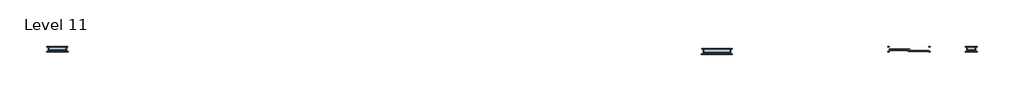
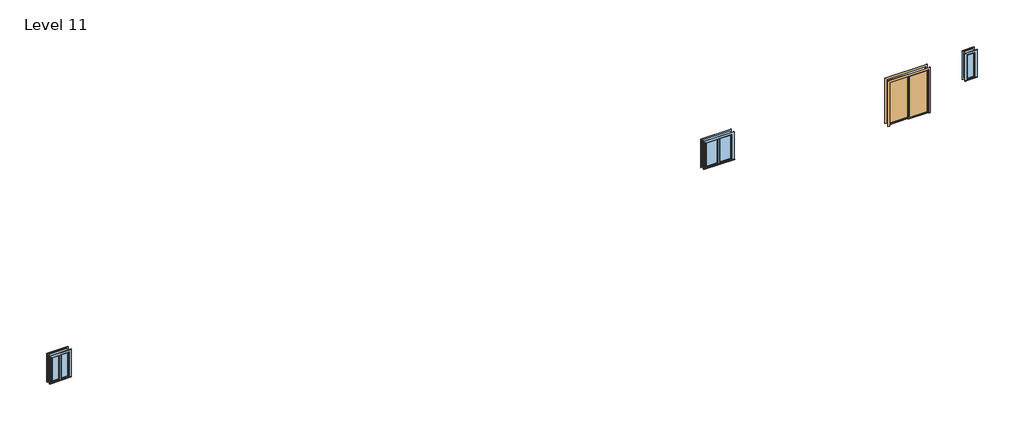
# One storey: 3 windows, 1 door.
"""IFC4 building model written with IfcOpenShell, lengths in millimetres."""

from ifc_helpers import new_model, si_unit, origin, place, context, project, spatial, transform, mapped, element, save
from components import door_076b30e0, window_a765b88f, window_bb17773d, window_0862ab64

model = new_model("IFC4")

# Units and contexts
model_context = context("Model", 3, world=origin())
ifc_project = project(units=[si_unit("LENGTHUNIT", "METRE", prefix="MILLI")], contexts=[model_context])

# Site, building, storey
site = spatial("IfcSite", under=ifc_project)
building = spatial("IfcBuilding", under=site)
storey = spatial("IfcBuildingStorey", under=building, Name="Level 11", Elevation=19507.2)

# Door
placement = place(None, origin())
door_shape = door_076b30e0(model_context)
element("IfcDoor", 1, ObjectType="Door-Double-Sliding : 68\" x 80\"", at=placement, inside=storey, context=model_context, shape_type="MappedRepresentation", body=[
    mapped(door_shape, transform((18530.214721, -12227.7237084, 19507.2), x_axis=(-1.0, 0.0, 0.0), y_axis=(0.0, -1.0, 0.0), z_axis=(0.0, 0.0, 1.0))),
])

# Windows
window_shape = window_a765b88f(model_context)
element("IfcWindow", 2, ObjectType="Awning with Trim : 16\" x 48\"", at=placement, inside=storey, context=model_context, shape_type="MappedRepresentation", body=[
    mapped(window_shape, transform((21273.414721, -12354.7237084, 19507.2), x_axis=(-1.0, 0.0, 0.0), y_axis=(0.0, -1.0, 0.0), z_axis=(0.0, 0.0, 1.0))),
])
window_2_shape = window_bb17773d(model_context)
element("IfcWindow", 3, ObjectType="Casement Dbl with Trim : 32\" x 48\"", at=placement, inside=storey, context=model_context, shape_type="MappedRepresentation", body=[
    mapped(window_2_shape, transform((-18960.185279, -12335.6737084, 19507.2), x_axis=(-1.0, 0.0, 0.0), y_axis=(0.0, -1.0, 0.0), z_axis=(0.0, 0.0, 1.0))),
])
window_3_shape = window_0862ab64(model_context)
element("IfcWindow", 4, ObjectType="Casement Dbl with Trim : 48\" x 48\"", at=placement, inside=storey, context=model_context, shape_type="MappedRepresentation", body=[
    mapped(window_3_shape, transform((10076.7594464, -12437.2737084, 19507.2), x_axis=(-1.0, 0.0, 0.0), y_axis=(0.0, -1.0, 0.0), z_axis=(0.0, 0.0, 1.0))),
])

save(model, "model.ifc")

# Revit data of these elements
# Type "Door-Double-Sliding : 68\" x 80\""
#   Type Mark = "10"
#   Construction Type Id = "opn-d45"
#   Assembly Code = "C1020"
#   Analytic Construction = "Wood frame, double glass door "
#   Thickness = 0' - 2"
#   Thermal Resistance (R) = 1.8150 (h·ft²·°F)/BTU
#   Heat Transfer Coefficient (U) = 0.5510 BTU/(h·ft²·°F)
#   Height = 6' - 8"
#   Rail Width = 0' - 2"
#   Stiles = 0' - 2"
#   Trim Projection Ext = 0' - 1"
#   Trim Projection Int = 0' - 1"
#   Trim Width = 0' - 3"
#   Width = 5' - 8"
#   Define Thermal Properties by = 1
#   Glazing = Glass
#   Panel Material = Wood - Birch - Solid Stained Light Low Gloss
#   Trim Material = Paint - Sienna
#   Visual Light Transmittance = 0
#   Solar Heat Gain Coefficient = 0
#   Function = (empty or 0)
#   Wall Closure = (empty or 0)
# Type "Awning with Trim : 16\" x 48\""
#   Type Mark = "14"
#   Construction Type Id = "GSP4R"
#   Assembly Code = "B2020100"
#   Analytic Construction = "1/8 in Pilkington single glazing"
#   Visual Light Transmittance = 0.9
#   Solar Heat Gain Coefficient = 0.78
#   Heat Transfer Coefficient (U) = 0.6496 BTU/(h·ft²·°F)
#   Height = 4' - 0"
#   Default Sill Height = 3' - 0"
#   Trim Projection - Ext. = 0' - 0 1/2"
#   Trim Projection - Int. = 0' - 0 3/4"
#   Trim Width - Exterior = 0' - 3 1/2"
#   Trim Width - Interior = 0' - 3 1/2"
#   Width = 1' - 4"
#   Window Inset = 0' - 0 3/4"
#   Define Thermal Properties by = 1
#   Glass Pane Material = Glass
#   Sash Material = Sash
#   Trim Exterior Material = Trim
#   Trim Interior Material = Trim
#   Wall Closure = (empty or 0)
# Type "Casement Dbl with Trim : 32\" x 48\""
#   Type Mark = "36"
#   Construction Type Id = "GSP4R"
#   Assembly Code = "B2020100"
#   Analytic Construction = "1/8 in Pilkington single glazing"
#   Visual Light Transmittance = 0.9
#   Solar Heat Gain Coefficient = 0.78
#   Heat Transfer Coefficient (U) = 0.6496 BTU/(h·ft²·°F)
#   Height = 4' - 0"
#   Default Sill Height = 3' - 0"
#   Trim Projection - Ext. = 0' - 0 1/2"
#   Trim Projection - Int. = 0' - 0 3/4"
#   Trim Width - Exterior = 0' - 3 1/2"
#   Trim Width - Interior = 0' - 3 1/2"
#   Width = 2' - 8"
#   Window Inset = 0' - 0 3/4"
#   Define Thermal Properties by = 1
#   Glass Pane Material = Glass
#   Sash Material = Sash
#   Trim Exterior Material = Trim
#   Trim Interior Material = Trim
#   Wall Closure = (empty or 0)
# Type "Casement Dbl with Trim : 48\" x 48\""
#   Type Mark = "34"
#   Construction Type Id = "GSP4R"
#   Assembly Code = "B2020100"
#   Analytic Construction = "1/8 in Pilkington single glazing"
#   Visual Light Transmittance = 0.9
#   Solar Heat Gain Coefficient = 0.78
#   Heat Transfer Coefficient (U) = 0.6496 BTU/(h·ft²·°F)
#   Height = 4' - 0"
#   Default Sill Height = 3' - 0"
#   Trim Projection - Ext. = 0' - 0 1/2"
#   Trim Projection - Int. = 0' - 0 3/4"
#   Trim Width - Exterior = 0' - 3 1/2"
#   Trim Width - Interior = 0' - 3 1/2"
#   Width = 4' - 0"
#   Window Inset = 0' - 0 3/4"
#   Define Thermal Properties by = 1
#   Glass Pane Material = Glass
#   Sash Material = Sash
#   Trim Exterior Material = Trim
#   Trim Interior Material = Trim
#   Wall Closure = (empty or 0)
# Element 1 (IfcDoor, "Door-Double-Sliding : 68\" x 80\"")
#   Phase Created = New Construction
#   Materials on its faces: "Paint - Sienna", "Wood - Birch - Solid Stained Light Low Gloss", "Glass"
# Element 2 (IfcWindow, "Awning with Trim : 16\" x 48\"")
#   Mark = "62"
#   Phase Created = New Construction
#   Materials on its faces: "Sash", "Trim", "Glass"
# Element 3 (IfcWindow, "Casement Dbl with Trim : 32\" x 48\"")
#   Mark = "45"
#   Phase Created = New Construction
#   Materials on its faces: "Sash", "Trim", "Glass"
# Element 4 (IfcWindow, "Casement Dbl with Trim : 48\" x 48\"")
#   Mark = "11"
#   Phase Created = New Construction
#   Materials on its faces: "Sash", "Trim", "Glass"
# Materials
#   "Glass": class "Glass", colour RGB 0 128 192, transparency 0.75, Description = "Soda Lime Glass", Cost = 0
#   "Wood - Birch - Solid Stained Light Low Gloss": class "Wood", colour RGB 210 159 95, transparency 0, Cost = 0
#   "Paint - Sienna": colour RGB 118 70 51, transparency 0, Cost = 0
#   "Sash": class "Wood", colour RGB 224 178 126, transparency 0
#   "Trim": class "Wood", colour RGB 224 178 126, transparency 0
